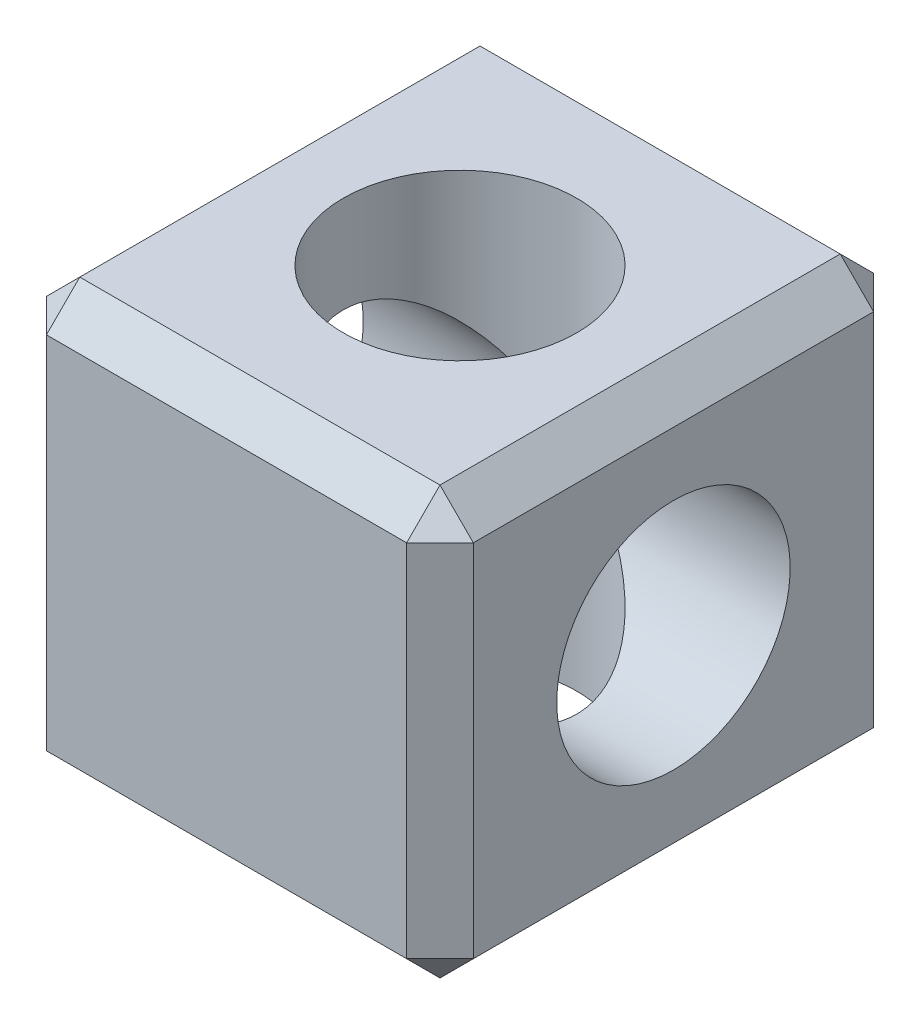
SolidWorks part; units mm, degrees
material "Plain Carbon Steel"
ref_plane "Front Plane" through (0, 0, 0) normal (0, 0, 1) x (1, 0, 0)
ref_plane "Top Plane" through (0, 0, 0) normal (0, 1, 0) x (1, 0, 0)
ref_plane "Right Plane" through (0, 0, 0) normal (1, 0, 0) x (0, 0, -1)
sketch "Block Profile Sketch" plane through (0, 0, 0) normal (0, 0, 1) x (1, 0, 0)
  line L1 (32, 32) -> (-32, 32)
  line L2 (32, 32) -> (32, -32)
  line L3 (32, -32) -> (-32, -32)
  line L4 (-32, 32) -> (-32, -32)
  line L5 (32, 32) -> (-32, -32) construction
  line L6 (32, -32) -> (-32, 32) construction
  point P0 (0, 0)
  dimension "D1" = 64
  dimension "D2" = 64
extrude "Block Body" add sketch "Block Profile Sketch" along normal blind 70
sketch "Cross Hole A Sketch" plane through (0, 32, 0) normal (0, 1, 0) x (1, 0, 0)
  line L0 (-32, -70) -> (-32, 0) construction
  circle A0 centre (0, -35) radius 17.5
  dimension "D1" = 35
  dimension "D2" = 35
  dimension "D3" = 32
extrude "Cross Hole A" cut sketch "Cross Hole A Sketch" against normal through all
sketch "Cross Hole B Sketch" plane through (32, 0, 0) normal (1, 0, 0) x (0, 0, -1)
  line L0 (0, -32) -> (0, 32) construction
  line L1 (-70, -32) -> (0, -32) construction
  circle A0 centre (-35, 0) radius 17.5
  dimension "D1" = 35
  dimension "D2" = 35
  dimension "D3" = 32
extrude "Cross Hole B" cut sketch "Cross Hole B Sketch" against normal through all
chamfer "Edge Chamfers 5x45°" distance 5 angle 45 11 edges at (-32, -32, 35) (-32, 0, 70) (0, -32, 70) (32, -32, 35) (32, 0, 70) (-32, 0, 0) (-32, 32, 35) (0, 32, 70) (32, 0, 0) (0, 32, 0) (32, 32, 35)
